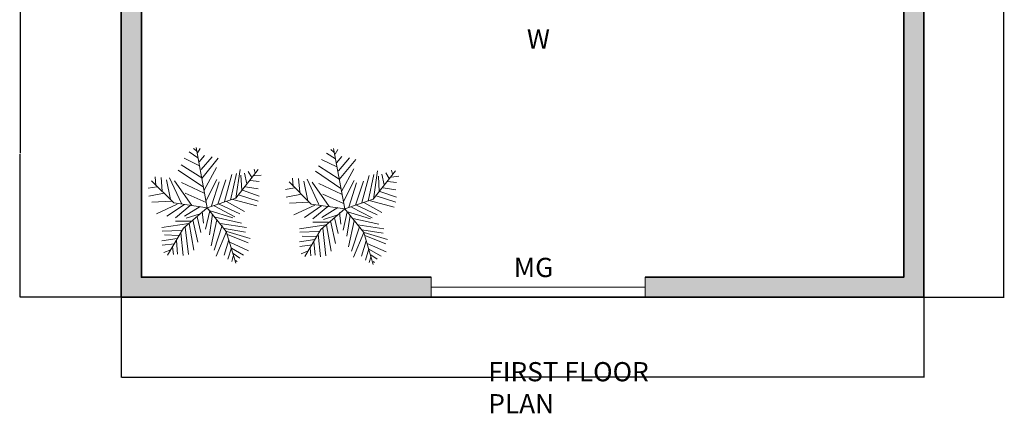
# Model space of a CAD drawing. Units: inches. Extents: x 1568 to 2529, y 2149 to 2897.
# Tile 14 of 16: x 2087 to 2529, y 2149 to 2326. Entities that reach past the tile are written whole.
import ezdxf

# ---------------------------------------------------------------- set-up
doc = ezdxf.new("R2010")
doc.units = ezdxf.units.IN
for name, color, linetype, lineweight in [('A-ANNO-DIMS', 2, 'Continuous', 18), ('A-DOOR', 4, 'Continuous', 18), ('A-WALL-PATT', 172, 'Continuous', 13), ('text', 210, 'Continuous', 18), ('TREE', 94, 'Continuous', 13), ('wall', 7, 'Continuous', 35)]:
    doc.layers.add(name, color=color, linetype=linetype, lineweight=lineweight)
doc.styles.get("Standard").update_dxf_attribs({"font": 'arial.ttf'})
doc.dimstyles.get("Standard").update_dxf_attribs({"dimtxt": 0.18, "dimasz": 0.18, "dimexe": 0.18, "dimexo": 0.0625, "dimgap": 0.09, "dimtad": 0, "dimtih": 1, "dimtoh": 1, "dimdec": 4, "dimzin": 0, "dimdsep": 46, "dimtxsty": 'Standard', "dimcen": 0.09, "dimadec": 0, "dimazin": 0, "dimtfac": 1, "dimtdec": 4, "dimtofl": 0, "dimtmove": 0, "dimatfit": 3, "dimfxl": 1, "dimtolj": 1, "dimtzin": 0, "dimarcsym": 0})

# ---------------------------------------------------------------- blocks, each defined once
blk = doc.blocks.new('*U10')
for p, q in [((-10.186, 53.64), (-13.084, 55.962)), ((0, 0), (-10.5, 57)), ((-9.099, 51.782), (-6.563, 55.962)), ((-7.288, 39.707), (-21.778, 46.673)), ((-8.737, 47.138), (-17.069, 52.711)), ((-7.65, 43.423), (-2.578, 49.46)), ((-5.839, 35.992), (4.667, 48.067)), ((-5.114, 27.632), (10.463, 46.673)), ((-5.114, 28.097), (-24.676, 40.636)), ((-2.941, 16.486), (8.652, 37.85)), ((-48.585, 21.131), (-49.309, 29.026)), ((-43.513, 28.561), (-42.427, 15.558)), ((-35.544, 28.097), (-24.314, 3.947)), ((-3.665, 19.273), (-27.574, 35.527)), ((16.259, 5.805), (23.142, 31.348)), ((22.055, 7.198), (27.489, 32.277)), ((27, 9), (48, 36)), ((27.127, 9.056), (31.112, 35.992)), ((31.836, 30.883), (32.561, 16.486)), ((35.096, 32.741), (37.27, 22.524)), ((38.719, 34.134), (41.979, 28.561)), ((43.791, 29.954), (51.036, 30.883)), ((44.153, 36.456), (45.239, 32.741)), ((-47.498, 19.737), (-55.83, 18.344)), ((-31.5, 4.5), (-52.5, 25.5)), ((-38.442, 26.239), (-34.819, 7.663)), ((-14.533, 2.09), (-30.834, 25.31)), ((-24.314, 23.917), (-2.941, 13.7)), ((-1.129, 6.734), (9.014, 26.704)), ((3.942, 1.625), (11.187, 24.381)), ((10.101, 3.483), (17.708, 26.239)), ((36.183, 19.737), (48.137, 17.88)), ((40.53, 25.775), (48.862, 24.846)), ((-40.615, 13.7), (-55.105, 10.913)), ((-20.691, 13.7), (-1.129, 4.876)), ((29.662, 12.307), (48.137, 6.269)), ((33.285, 16.486), (48.862, 10.913)), ((-33.37, 6.269), (-52.207, 5.34)), ((-28.299, 3.483), (-47.86, -5.805)), ((-21.416, 3.018), (-38.079, -8.128)), ((0, 0), (-31.5, 4.5)), ((-15.982, 2.09), (-30.11, -9.521)), ((0, 0), (-22.5, -19.5)), ((-6.563, 1.161), (-21.416, -8.128)), ((0, 0), (27, 9)), ((0, 0), (18, -22.5)), ((6.478, 1.625), (26.04, -8.592)), ((11.187, 3.483), (30.749, -5.805)), ((18.07, 5.805), (35.096, -3.483)), ((24.229, 7.663), (46.688, 1.625)), ((-6.563, -5.805), (-19.967, -9.985)), ((-9.461, -8.592), (-6.201, -23.453)), ((-4.752, -3.483), (-3.665, -14.629)), ((2.493, -3.019), (-1.491, -20.202)), ((1.769, -2.555), (24.229, -9.521)), ((5.029, -6.27), (2.131, -25.775)), ((7.565, -9.056), (32.198, -14.629)), ((-17.431, -15.094), (-42.789, -18.809)), ((-15.257, -12.772), (-30.11, -12.772)), ((-20.691, -18.345), (-17.793, -44.352)), ((-17.069, -15.094), (-12.721, -40.172)), ((-13.446, -11.378), (-8.737, -32.741)), ((9.014, -11.378), (3.58, -35.992)), ((14.085, -16.951), (6.478, -40.172)), ((12.274, -15.094), (36.907, -18.809)), ((-24.314, -21.596), (-42.427, -22.06)), ((-26.849, -26.24), (-40.253, -25.775)), ((-22.5, -19.5), (-37.5, -45)), ((-25.038, -23.918), (-22.865, -45.281)), ((18.07, -22.524), (8.289, -45.745)), ((16.259, -19.738), (36.183, -22.989)), ((18, -22.5), (27, -52.5)), ((18.433, -22.524), (40.53, -29.026)), ((19.157, -25.311), (38.719, -33.206)), ((-28.299, -29.026), (-42.789, -31.348)), ((-30.834, -34.135), (-42.427, -35.528)), ((-32.646, -36.921), (-31.921, -44.352)), ((-29.023, -30.884), (-27.936, -43.887)), ((20.244, -30.419), (15.897, -44.816)), ((21.331, -32.741), (39.081, -40.636)), ((-34.457, -39.708), (-40.978, -42.494)), ((22.78, -37.85), (19.519, -48.532)), ((22.78, -38.314), (34.372, -44.816)), ((24.591, -45.745), (23.142, -50.854)), ((24.591, -43.423), (30.749, -47.603)), ((26.764, -49.925), (28.213, -50.854))]:
    blk.add_line(p, q)
blk = doc.blocks.new('*D37')
at = {"layer": 'A-ANNO-DIMS', "color": 0, "lineweight": -2, "transparency": 16777216}
for p, q in [((2132.85, 2201.47), (2132.85, 2165.5)), ((2492.85, 2201.47), (2492.85, 2165.5)), ((2133.03, 2165.68), (2312.56, 2165.68)), ((2492.67, 2165.68), (2313.14, 2165.68))]:
    blk.add_line(p, q, dxfattribs=at)
at = {"layer": 'A-ANNO-DIMS', "color": 0, "transparency": 16777216}
for points in [[(2133.03, 2165.71), (2133.03, 2165.65), (2132.85, 2165.68)], [(2492.67, 2165.71), (2492.67, 2165.65), (2492.85, 2165.68)]]:
    blk.add_solid(points, dxfattribs=at)
at = {"layer": 'Defpoints', "color": 0, "transparency": 16777216}
for p in [(2132.85, 2201.53), (2492.85, 2201.53), (2492.85, 2165.68)]:
    blk.add_point(p, dxfattribs=at)
at = {"layer": 'A-ANNO-DIMS', "color": 0, "transparency": 16777216, "insert": (2312.85, 2165.68), "char_height": 0.18, "attachment_point": 5}
blk.add_mtext('\\A1;360', dxfattribs=at)
blk = doc.blocks.new('*D38')
at = {"layer": 'A-ANNO-DIMS', "color": 0, "lineweight": -2, "transparency": 16777216}
for p, q in [((2492.94, 2801.53), (2528.91, 2801.53)), ((2528.73, 2801.35), (2528.73, 2501.71)), ((2528.73, 2201.71), (2528.73, 2501.35)), ((2492.91, 2201.53), (2528.91, 2201.53))]:
    blk.add_line(p, q, dxfattribs=at)
at = {"layer": 'A-ANNO-DIMS', "color": 0, "transparency": 16777216}
for points in [[(2528.7, 2801.35), (2528.76, 2801.35), (2528.73, 2801.53)], [(2528.7, 2201.71), (2528.76, 2201.71), (2528.73, 2201.53)]]:
    blk.add_solid(points, dxfattribs=at)
at = {"layer": 'Defpoints', "color": 0, "transparency": 16777216}
for p in [(2492.88, 2801.53), (2528.73, 2801.53), (2492.85, 2201.53)]:
    blk.add_point(p, dxfattribs=at)
at = {"layer": 'A-ANNO-DIMS', "color": 0, "transparency": 16777216, "insert": (2528.73, 2501.53), "char_height": 0.18, "attachment_point": 5}
blk.add_mtext('\\A1;600', dxfattribs=at)
blk = doc.blocks.new('*D39')
at = {"layer": 'A-ANNO-DIMS', "color": 0, "lineweight": -2, "transparency": 16777216}
for p, q in [((2132.79, 2330.53), (2087.29, 2330.53)), ((2087.47, 2330.35), (2087.47, 2266.21)), ((2087.47, 2201.71), (2087.47, 2265.85)), ((2132.79, 2201.53), (2087.29, 2201.53))]:
    blk.add_line(p, q, dxfattribs=at)
at = {"layer": 'A-ANNO-DIMS', "color": 0, "transparency": 16777216}
for points in [[(2087.44, 2330.35), (2087.5, 2330.35), (2087.47, 2330.53)], [(2087.44, 2201.71), (2087.5, 2201.71), (2087.47, 2201.53)]]:
    blk.add_solid(points, dxfattribs=at)
at = {"layer": 'Defpoints', "color": 0, "transparency": 16777216}
for p in [(2087.47, 2330.53), (2132.85, 2330.53), (2132.85, 2201.53)]:
    blk.add_point(p, dxfattribs=at)
at = {"layer": 'A-ANNO-DIMS', "color": 0, "transparency": 16777216, "insert": (2087.47, 2266.03), "char_height": 0.18, "attachment_point": 5}
blk.add_mtext('\\A1;129', dxfattribs=at)

msp = doc.modelspace()

# ---------------------------------------------------------------- hatches: boundary and pattern name
at = {"layer": 'A-WALL-PATT'}
h = msp.add_hatch(color=256, dxfattribs=at)
h.dxf.hatch_style = 1
h.paths.add_polyline_path([(2257.4593, 2801.532), (2153.7841, 2801.532), (2153.7841, 2792.532), (2257.4593, 2792.532)])
h.paths.add_polyline_path([(2331.7115, 2801.532), (2278.3925, 2801.532), (2278.3925, 2792.532), (2331.7115, 2792.532)])
h.paths.add_polyline_path([(2141.8509, 2753.3576), (2141.6865, 2753.3576), (2132.8509, 2753.3576), (2132.8509, 2705.9172), (2141.8509, 2705.9172)])
h.paths.add_polyline_path([(2278.3509, 2757.9833), (2274.1052, 2757.9833, -0.00224577), (2273.8509, 2757.9844), (2273.8509, 2744.532), (2141.8509, 2744.532), (2141.8509, 2740.032), (2273.8509, 2740.032), (2273.8509, 2730.8156), (2278.3509, 2730.8156), (2278.3509, 2740.032)])
h.paths.add_polyline_path([(2471.947, 2801.532), (2367.7115, 2801.532), (2367.7115, 2792.532), (2471.947, 2792.532)])
h.paths.add_polyline_path([(2402.7886, 2351.2573), (2436.5067, 2351.2573), (2436.5067, 2383.453), (2402.7886, 2383.453)], flags=9)
h.paths.add_polyline_path([(2363.115, 2703.2844), (2384.1733, 2703.2844), (2384.1733, 2721.0645), (2363.115, 2721.0645)], flags=9)
h.paths.add_polyline_path([(2367.7631, 2584.032), (2380.7818, 2584.032), (2380.7818, 2601.8121), (2367.7631, 2601.8121)], flags=9)
h.paths.add_polyline_path([(2412.2706, 2522.1491), (2473.8683, 2522.1491), (2473.8683, 2568.725), (2412.2706, 2568.725)], flags=9)
h.paths.add_polyline_path([(2412.2706, 2686.5293), (2474.6569, 2686.5293), (2474.6569, 2718.725), (2412.2706, 2718.725)], flags=9)
h.paths.add_polyline_path([(2305.8704, 2205.7429), (2329.6007, 2205.7429), (2329.6007, 2223.523), (2305.8704, 2223.523)], flags=9)
h.paths.add_polyline_path([(2312.4696, 2308.5242), (2328.1604, 2308.5242), (2328.1604, 2326.3043), (2312.4696, 2326.3043)], flags=9)
h.paths.add_polyline_path([(2253.7912, 2420.5203), (2266.8099, 2420.5203), (2266.8099, 2438.3004), (2253.7912, 2438.3004)], flags=9)
h.paths.add_polyline_path([(2261.5714, 2703.4315), (2274.5902, 2703.4315), (2274.5902, 2721.2116), (2261.5714, 2721.2116)], flags=9)
h.paths.add_polyline_path([(2277.898, 2569.2764), (2333.9221, 2569.2764), (2333.9221, 2601.4721), (2277.898, 2601.4721)], flags=9)
h.paths.add_polyline_path([(2176.0749, 2419.8331), (2231.9754, 2419.8331), (2231.9754, 2452.0288), (2176.0749, 2452.0288)], flags=9)
h.paths.add_polyline_path([(2213.9423, 2525.7697), (2252.2216, 2525.7697), (2252.2216, 2557.9653), (2213.9423, 2557.9653)], flags=9)
h.paths.add_polyline_path([(2170.6878, 2692.4783), (2211.1801, 2692.4783), (2211.1801, 2724.6739), (2170.6878, 2724.6739)], flags=9)
h.paths.add_polyline_path([(2262.4629, 2764.5694), (2275.4816, 2764.5694), (2275.4816, 2782.3495), (2262.4629, 2782.3495)], flags=9)
h.paths.add_polyline_path([(2183.6493, 2749.7187), (2217.3673, 2749.7187), (2217.3673, 2781.9143), (2183.6493, 2781.9143)], flags=9)
h = msp.add_hatch(color=256, dxfattribs=at)
h.dxf.hatch_style = 1
h.paths.add_polyline_path([(2492.8509, 2792.532), (2483.8509, 2792.532), (2483.8509, 2699.1671), (2492.8509, 2699.1671)])
h.paths.add_polyline_path([(2278.3509, 2690.8156), (2273.8509, 2690.8156), (2273.8509, 2624.532), (2278.3509, 2624.532)])
h.paths.add_polyline_path([(2257.4177, 2620.032), (2153.7841, 2620.032), (2153.7841, 2615.532), (2257.4177, 2615.532)])
h.paths.add_polyline_path([(2141.8509, 2669.9172), (2132.8509, 2669.9172), (2132.8509, 2624.532), (2141.8509, 2624.532)])
h.paths.add_polyline_path([(2402.7886, 2351.2573), (2436.5067, 2351.2573), (2436.5067, 2383.453), (2402.7886, 2383.453)], flags=9)
h.paths.add_polyline_path([(2363.115, 2703.2844), (2384.1733, 2703.2844), (2384.1733, 2721.0645), (2363.115, 2721.0645)], flags=9)
h.paths.add_polyline_path([(2367.7631, 2584.032), (2380.7818, 2584.032), (2380.7818, 2601.8121), (2367.7631, 2601.8121)], flags=9)
h.paths.add_polyline_path([(2412.2706, 2522.1491), (2473.8683, 2522.1491), (2473.8683, 2568.725), (2412.2706, 2568.725)], flags=9)
h.paths.add_polyline_path([(2412.2706, 2686.5293), (2474.6569, 2686.5293), (2474.6569, 2718.725), (2412.2706, 2718.725)], flags=9)
h.paths.add_polyline_path([(2305.8704, 2205.7429), (2329.6007, 2205.7429), (2329.6007, 2223.523), (2305.8704, 2223.523)], flags=9)
h.paths.add_polyline_path([(2312.4696, 2308.5242), (2328.1604, 2308.5242), (2328.1604, 2326.3043), (2312.4696, 2326.3043)], flags=9)
h.paths.add_polyline_path([(2253.7912, 2420.5203), (2266.8099, 2420.5203), (2266.8099, 2438.3004), (2253.7912, 2438.3004)], flags=9)
h.paths.add_polyline_path([(2261.5714, 2703.4315), (2274.5902, 2703.4315), (2274.5902, 2721.2116), (2261.5714, 2721.2116)], flags=9)
h.paths.add_polyline_path([(2262.4629, 2764.5694), (2275.4816, 2764.5694), (2275.4816, 2782.3495), (2262.4629, 2782.3495)], flags=9)
h.paths.add_polyline_path([(2277.898, 2569.2764), (2333.9221, 2569.2764), (2333.9221, 2601.4721), (2277.898, 2601.4721)], flags=9)
h.paths.add_polyline_path([(2176.0749, 2419.8331), (2231.9754, 2419.8331), (2231.9754, 2452.0288), (2176.0749, 2452.0288)], flags=9)
h.paths.add_polyline_path([(2213.9423, 2525.7697), (2252.2216, 2525.7697), (2252.2216, 2557.9653), (2213.9423, 2557.9653)], flags=9)
h.paths.add_polyline_path([(2170.6878, 2692.4783), (2211.1801, 2692.4783), (2211.1801, 2724.6739), (2170.6878, 2724.6739)], flags=9)
h.paths.add_polyline_path([(2183.6493, 2749.7187), (2217.3673, 2749.7187), (2217.3673, 2781.9143), (2183.6493, 2781.9143)], flags=9)
h = msp.add_hatch(color=256, dxfattribs=at)
h.dxf.hatch_style = 1
h.paths.add_polyline_path([(2141.8509, 2615.532), (2132.8509, 2615.532), (2132.8509, 2564.2764), (2141.8509, 2564.2764)])
h.paths.add_polyline_path([(2141.8509, 2528.2764), (2132.8509, 2528.2764), (2132.8509, 2436.512), (2141.8509, 2436.512), (2141.8509, 2459.532)])
h.paths.add_polyline_path([(2278.3509, 2464.032), (2253.6925, 2464.032), (2141.8509, 2464.032), (2141.8509, 2459.532), (2255.8509, 2459.532), (2273.8509, 2459.532), (2273.8509, 2451.2271), (2278.3509, 2451.2271)])
h.paths.add_polyline_path([(2141.8509, 2400.512), (2132.8509, 2400.512), (2132.8509, 2339.532), (2141.8509, 2339.532)])
h.paths.add_polyline_path([(2258.2144, 2339.532), (2153.7841, 2339.532), (2153.7841, 2330.532), (2258.2144, 2330.532)])
h.paths.add_polyline_path([(2291.8353, 2339.532), (2279.1476, 2339.532), (2279.1476, 2330.532), (2291.8353, 2330.532)])
h.paths.add_polyline_path([(2402.7886, 2351.2573), (2436.5067, 2351.2573), (2436.5067, 2383.453), (2402.7886, 2383.453)], flags=9)
h.paths.add_polyline_path([(2363.115, 2703.2844), (2384.1733, 2703.2844), (2384.1733, 2721.0645), (2363.115, 2721.0645)], flags=9)
h.paths.add_polyline_path([(2367.7631, 2584.032), (2380.7818, 2584.032), (2380.7818, 2601.8121), (2367.7631, 2601.8121)], flags=9)
h.paths.add_polyline_path([(2412.2706, 2522.1491), (2473.8683, 2522.1491), (2473.8683, 2568.725), (2412.2706, 2568.725)], flags=9)
h.paths.add_polyline_path([(2412.2706, 2686.5293), (2474.6569, 2686.5293), (2474.6569, 2718.725), (2412.2706, 2718.725)], flags=9)
h.paths.add_polyline_path([(2305.8704, 2205.7429), (2329.6007, 2205.7429), (2329.6007, 2223.523), (2305.8704, 2223.523)], flags=9)
h.paths.add_polyline_path([(2312.4696, 2308.5242), (2328.1604, 2308.5242), (2328.1604, 2326.3043), (2312.4696, 2326.3043)], flags=9)
h.paths.add_polyline_path([(2261.5714, 2703.4315), (2274.5902, 2703.4315), (2274.5902, 2721.2116), (2261.5714, 2721.2116)], flags=9)
h.paths.add_polyline_path([(2262.4629, 2764.5694), (2275.4816, 2764.5694), (2275.4816, 2782.3495), (2262.4629, 2782.3495)], flags=9)
h.paths.add_polyline_path([(2277.898, 2569.2764), (2333.9221, 2569.2764), (2333.9221, 2601.4721), (2277.898, 2601.4721)], flags=9)
h.paths.add_polyline_path([(2213.9423, 2525.7697), (2252.2216, 2525.7697), (2252.2216, 2557.9653), (2213.9423, 2557.9653)], flags=9)
h.paths.add_polyline_path([(2170.6878, 2692.4783), (2211.1801, 2692.4783), (2211.1801, 2724.6739), (2170.6878, 2724.6739)], flags=9)
h.paths.add_polyline_path([(2183.6493, 2749.7187), (2217.3673, 2749.7187), (2217.3673, 2781.9143), (2183.6493, 2781.9143)], flags=9)
h = msp.add_hatch(color=256, dxfattribs=at)
h.dxf.hatch_style = 1
h.paths.add_polyline_path([(2492.8509, 2663.1671), (2483.8509, 2663.1671), (2483.8509, 2630.5978), (2492.8509, 2630.5978)])
h.paths.add_polyline_path([(2492.8509, 2609.6646), (2483.8509, 2609.6646), (2483.8509, 2572.3679), (2492.8509, 2572.3679)])
h.paths.add_polyline_path([(2492.8509, 2536.3679), (2483.8509, 2536.3679), (2483.8509, 2476.032), (2483.8509, 2458.371), (2492.8509, 2458.371)])
h.paths.add_polyline_path([(2483.8509, 2620.032), (2361.425, 2620.032), (2359.3509, 2620.032), (2359.3509, 2607.8035), (2363.8509, 2607.8035), (2363.8509, 2615.532), (2483.8509, 2615.532)])
h.paths.add_polyline_path([(2402.7886, 2351.2573), (2436.5067, 2351.2573), (2436.5067, 2383.453), (2402.7886, 2383.453)], flags=9)
h.paths.add_polyline_path([(2412.2706, 2522.1491), (2473.8683, 2522.1491), (2473.8683, 2568.725), (2412.2706, 2568.725)], flags=9)
h.paths.add_polyline_path([(2305.8704, 2205.7429), (2329.6007, 2205.7429), (2329.6007, 2223.523), (2305.8704, 2223.523)], flags=9)
h.paths.add_polyline_path([(2312.4696, 2308.5242), (2328.1604, 2308.5242), (2328.1604, 2326.3043), (2312.4696, 2326.3043)], flags=9)
h.paths.add_polyline_path([(2253.7912, 2420.5203), (2266.8099, 2420.5203), (2266.8099, 2438.3004), (2253.7912, 2438.3004)], flags=9)
h.paths.add_polyline_path([(2261.5714, 2703.4315), (2274.5902, 2703.4315), (2274.5902, 2721.2116), (2261.5714, 2721.2116)], flags=9)
h.paths.add_polyline_path([(2262.4629, 2764.5694), (2275.4816, 2764.5694), (2275.4816, 2782.3495), (2262.4629, 2782.3495)], flags=9)
h.paths.add_polyline_path([(2277.898, 2569.2764), (2333.9221, 2569.2764), (2333.9221, 2601.4721), (2277.898, 2601.4721)], flags=9)
h.paths.add_polyline_path([(2176.0749, 2419.8331), (2231.9754, 2419.8331), (2231.9754, 2452.0288), (2176.0749, 2452.0288)], flags=9)
h.paths.add_polyline_path([(2213.9423, 2525.7697), (2252.2216, 2525.7697), (2252.2216, 2557.9653), (2213.9423, 2557.9653)], flags=9)
h.paths.add_polyline_path([(2170.6878, 2692.4783), (2211.1801, 2692.4783), (2211.1801, 2724.6739), (2170.6878, 2724.6739)], flags=9)
h.paths.add_polyline_path([(2183.6493, 2749.7187), (2217.3673, 2749.7187), (2217.3673, 2781.9143), (2183.6493, 2781.9143)], flags=9)
h = msp.add_hatch(color=256, dxfattribs=at)
h.dxf.hatch_style = 1
h.paths.add_polyline_path([(2492.8509, 2422.371), (2483.8509, 2422.371), (2483.8509, 2339.532), (2492.8509, 2339.532)])
h.paths.add_polyline_path([(2483.8509, 2416.032), (2464.9258, 2416.032), (2464.9258, 2411.7863), (2464.9258, 2411.532), (2483.8509, 2411.532)])
h.paths.add_polyline_path([(2402.7886, 2351.2573), (2436.5067, 2351.2573), (2436.5067, 2383.453), (2402.7886, 2383.453)], flags=9)
h.paths.add_polyline_path([(2363.115, 2703.2844), (2384.1733, 2703.2844), (2384.1733, 2721.0645), (2363.115, 2721.0645)], flags=9)
h.paths.add_polyline_path([(2367.7631, 2584.032), (2380.7818, 2584.032), (2380.7818, 2601.8121), (2367.7631, 2601.8121)], flags=9)
h.paths.add_polyline_path([(2412.2706, 2522.1491), (2473.8683, 2522.1491), (2473.8683, 2568.725), (2412.2706, 2568.725)], flags=9)
h.paths.add_polyline_path([(2412.2706, 2686.5293), (2474.6569, 2686.5293), (2474.6569, 2718.725), (2412.2706, 2718.725)], flags=9)
h.paths.add_polyline_path([(2305.8704, 2205.7429), (2329.6007, 2205.7429), (2329.6007, 2223.523), (2305.8704, 2223.523)], flags=9)
h.paths.add_polyline_path([(2312.4696, 2308.5242), (2328.1604, 2308.5242), (2328.1604, 2326.3043), (2312.4696, 2326.3043)], flags=9)
h.paths.add_polyline_path([(2253.7912, 2420.5203), (2266.8099, 2420.5203), (2266.8099, 2438.3004), (2253.7912, 2438.3004)], flags=9)
h.paths.add_polyline_path([(2261.5714, 2703.4315), (2274.5902, 2703.4315), (2274.5902, 2721.2116), (2261.5714, 2721.2116)], flags=9)
h.paths.add_polyline_path([(2262.4629, 2764.5694), (2275.4816, 2764.5694), (2275.4816, 2782.3495), (2262.4629, 2782.3495)], flags=9)
h.paths.add_polyline_path([(2277.898, 2569.2764), (2333.9221, 2569.2764), (2333.9221, 2601.4721), (2277.898, 2601.4721)], flags=9)
h.paths.add_polyline_path([(2176.0749, 2419.8331), (2231.9754, 2419.8331), (2231.9754, 2452.0288), (2176.0749, 2452.0288)], flags=9)
h.paths.add_polyline_path([(2213.9423, 2525.7697), (2252.2216, 2525.7697), (2252.2216, 2557.9653), (2213.9423, 2557.9653)], flags=9)
h.paths.add_polyline_path([(2170.6878, 2692.4783), (2211.1801, 2692.4783), (2211.1801, 2724.6739), (2170.6878, 2724.6739)], flags=9)
h.paths.add_polyline_path([(2183.6493, 2749.7187), (2217.3673, 2749.7187), (2217.3673, 2781.9143), (2183.6493, 2781.9143)], flags=9)
h = msp.add_hatch(color=256, dxfattribs=at)
h.dxf.hatch_style = 1
h.paths.add_polyline_path([(2436.6209, 2416.032), (2363.8509, 2416.032), (2363.8509, 2411.532), (2436.6209, 2411.532)])
h.paths.add_polyline_path([(2363.115, 2703.2844), (2384.1733, 2703.2844), (2384.1733, 2721.0645), (2363.115, 2721.0645)], flags=9)
h.paths.add_polyline_path([(2367.7631, 2584.032), (2380.7818, 2584.032), (2380.7818, 2601.8121), (2367.7631, 2601.8121)], flags=9)
h.paths.add_polyline_path([(2412.2706, 2522.1491), (2473.8683, 2522.1491), (2473.8683, 2568.725), (2412.2706, 2568.725)], flags=9)
h.paths.add_polyline_path([(2412.2706, 2686.5293), (2474.6569, 2686.5293), (2474.6569, 2718.725), (2412.2706, 2718.725)], flags=9)
h.paths.add_polyline_path([(2261.5714, 2703.4315), (2274.5902, 2703.4315), (2274.5902, 2721.2116), (2261.5714, 2721.2116)], flags=9)
h.paths.add_polyline_path([(2262.4629, 2764.5694), (2275.4816, 2764.5694), (2275.4816, 2782.3495), (2262.4629, 2782.3495)], flags=9)
h.paths.add_polyline_path([(2277.898, 2569.2764), (2333.9221, 2569.2764), (2333.9221, 2601.4721), (2277.898, 2601.4721)], flags=9)
h.paths.add_polyline_path([(2213.9423, 2525.7697), (2252.2216, 2525.7697), (2252.2216, 2557.9653), (2213.9423, 2557.9653)], flags=9)
h.paths.add_polyline_path([(2170.6878, 2692.4783), (2211.1801, 2692.4783), (2211.1801, 2724.6739), (2170.6878, 2724.6739)], flags=9)
h.paths.add_polyline_path([(2183.6493, 2749.7187), (2217.3673, 2749.7187), (2217.3673, 2781.9143), (2183.6493, 2781.9143)], flags=9)
h.paths.add_polyline_path([(2402.7886, 2351.2573), (2436.5067, 2351.2573), (2436.5067, 2383.453), (2402.7886, 2383.453)], flags=9)
h.paths.add_polyline_path([(2305.8704, 2205.7429), (2329.6007, 2205.7429), (2329.6007, 2223.523), (2305.8704, 2223.523)], flags=9)
h.paths.add_polyline_path([(2312.4696, 2308.5242), (2328.1604, 2308.5242), (2328.1604, 2326.3043), (2312.4696, 2326.3043)], flags=9)
h.paths.add_polyline_path([(2253.7912, 2420.5203), (2266.8099, 2420.5203), (2266.8099, 2438.3004), (2253.7912, 2438.3004)], flags=9)
h.paths.add_polyline_path([(2176.0749, 2419.8331), (2231.9754, 2419.8331), (2231.9754, 2452.0288), (2176.0749, 2452.0288)], flags=9)
h = msp.add_hatch(color=256, dxfattribs=at)
h.dxf.hatch_style = 1
h.paths.add_polyline_path([(2492.8509, 2330.532), (2483.8509, 2330.532), (2483.8509, 2210.532), (2367.8146, 2210.532), (2367.8146, 2201.532), (2492.8509, 2201.532)])
h.paths.add_polyline_path([(2141.8509, 2330.532), (2132.8509, 2330.532), (2132.8509, 2201.532), (2271.818, 2201.532), (2271.818, 2210.532), (2141.8509, 2210.532)])

# ---------------------------------------------------------------- linework, layer by layer
at = {"layer": 'A-DOOR'}
for p, q in [((2271.818, 2210.532), (2271.818, 2201.532)), ((2367.8146, 2210.532), (2367.8146, 2201.532)), ((2271.818, 2206.032), (2367.8146, 2206.032))]:
    msp.add_line(p, q, dxfattribs=at)
at = {"layer": 'wall'}
msp.add_line((2141.8509, 2210.532), (2141.8509, 2330.532), dxfattribs=at)
msp.add_lwpolyline([(2132.8509, 2201.532), (2492.8509, 2201.532), (2492.8509, 2801.532), (2132.8509, 2801.532)], close=True, dxfattribs=at)
for points in [[(2141.8509, 2330.532), (2141.8509, 2210.532), (2271.818, 2210.532)], [(2367.8146, 2210.532), (2483.8509, 2210.532), (2483.8509, 2330.532)]]:
    msp.add_lwpolyline(points, dxfattribs=at)

# ---------------------------------------------------------------- block references
at = {"layer": 'TREE', "xscale": 0.4751991687393962, "yscale": 0.4751991687393962, "zscale": 0.4751991687393962}
for p in [(2171.3905, 2241.7484), (2233.0402, 2241.2541)]:
    msp.add_blockref('*U10', p, dxfattribs=at)

# ---------------------------------------------------------------- texts
at = {"layer": 'text', "attachment_point": 1}
for s, heights, insert, char_height in [('W', [23.0437], (2314.7738, 2321.8637), 8.6281), ('MG', [23.0437], (2308.922, 2219.2295), 8.62815), ('FIRST FLOOR PLAN', [0], (2297.4839, 2172.397), 8.628146)]:
    msp.add_mtext_dynamic_manual_height_columns(s, width=94.297369, gutter_width=43.1407, heights=heights, dxfattribs=dict(at, insert=insert, char_height=char_height))

# ---------------------------------------------------------------- dimensions: what is measured, and where the dimension line sits
at = {"layer": 'A-ANNO-DIMS'}
for base, p1, p2, picture, middle in [((2528.7302, 2801.532), (2492.8509, 2201.532), (2492.8802, 2801.532), '*D38', (2528.7302, 2501.532)), ((2087.4667, 2330.532), (2132.8509, 2201.532), (2132.8509, 2330.532), '*D39', (2087.4667, 2266.032))]:
    dim = msp.add_linear_dim(base=base, p1=p1, p2=p2, angle=90, dimstyle='Standard', override={"dimdec": 0, "dimlfac": 1, "dimrnd": 0, "dimzin": 0, "dimdsep": 46, "dimlunit": 2}, dxfattribs=at)
    dim.commit()
    dim.dimension.update_dxf_attribs({"geometry": picture, "text_midpoint": middle})
dim = msp.add_linear_dim(base=(2492.8509, 2165.682), p1=(2132.8509, 2201.532), p2=(2492.8509, 2201.532), dimstyle='Standard', override={"dimdec": 0, "dimlfac": 1, "dimrnd": 0, "dimzin": 0, "dimdsep": 46, "dimlunit": 2}, dxfattribs=at)
dim.commit()
dim.dimension.update_dxf_attribs({"geometry": '*D37', "text_midpoint": (2312.8509, 2165.682)})

doc.saveas('drawing.dxf')
